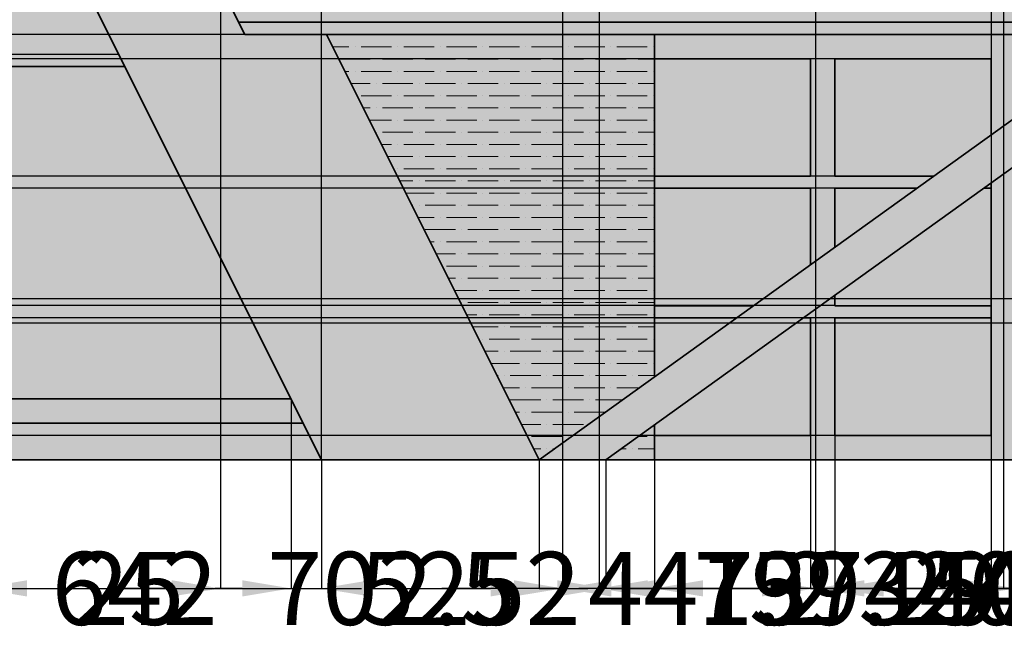
# Model space of a CAD drawing. Units: millimetres. Extents: x -504 to 6314, y 1290 to 4335.
# Tile 3 of 9: x 1774 to 3796, y 1290 to 2556. Entities that reach past the tile are written whole.
import ezdxf

# ---------------------------------------------------------------- set-up
doc = ezdxf.new("R2010")
doc.units = ezdxf.units.MM
doc.header["$MEASUREMENT"] = 0
for name, color, linetype, lineweight in [('A-ANNO-DIMS', 2, 'Continuous', 18), ('A-ELEV', 7, 'Continuous', 35), ('A-ELEV-PATT', 8, 'Continuous', 13)]:
    doc.layers.add(name, color=color, linetype=linetype, lineweight=lineweight)
doc.styles.get("Standard").update_dxf_attribs({"font": 'arial.ttf'})
doc.dimstyles.get("Standard").update_dxf_attribs({"dimtxt": 150, "dimasz": 100, "dimexe": 0.18, "dimexo": 0.0625, "dimgap": 0.09, "dimtad": 0, "dimtih": 1, "dimtoh": 1, "dimdec": 0, "dimzin": 0, "dimdsep": 46, "dimtxsty": 'Standard', "dimcen": 0.09, "dimadec": 0, "dimazin": 0, "dimtfac": 1, "dimtdec": 0, "dimtofl": 0, "dimtmove": 0, "dimatfit": 3, "dimfxl": 1, "dimtolj": 1, "dimtzin": 0, "dimarcsym": 0})
pattern_1 = [(50, (0, 0), (71.726, -6.2752), [7.5, -82.5]), (355, (0, 0), (-13.8751, 75.2192), [6, -66]), (100.4514, (5.98, -0.52), (57.8509, 68.944), [6.374, -70.1142]), (46.1842, (0, 20), (106.7241, -16.5519), [11.25, -123.75]), (96.6356, (8.89, 18.62), (93.4662, 97.4119), [9.561, -105.1714]), (351.1842, (0, 20), (93.4662, 97.4119), [9, -99]), (21, (10, 15), (59.6907, -40.2619), [7.5, -82.5]), (326, (10, 15), (24.3315, 72.515), [6, -66]), (71.4514, (14.974, 11.645), (84.0222, 32.2531), [6.374, -70.1142]), (37.5, (0, 0), (1.21599, 33.28939), [0, -65.2, 0, -67, 0, -66.25]), (7.5, (0, 0), (26.30695, 39.44117), [0, -38.2, 0, -63.7, 0, -25.25]), (327.5, (-22.3, 0), (53.38224, -2.25549), [0, -25, 0, -78, 0, -103.5]), (317.5, (-32.3, 0), (58.3186, 10.0105), [0, -32.5, 0, -51.8, 0, -73.5])]

# ---------------------------------------------------------------- blocks, each defined once
blk = doc.blocks.new('*D1')
at = {"layer": 'A-ANNO-DIMS', "color": 0, "lineweight": -2, "transparency": 16777216}
for p, q in [((5324.8, 2261.1), (5324.8, 1387.9)), ((72.8, 1652.1), (72.8, 1387.9)), ((172.8, 1388.1), (2475.5, 1388.1)), ((5224.8, 1388.1), (2922.1, 1388.1))]:
    blk.add_line(p, q, dxfattribs=at)
at = {"layer": 'A-ANNO-DIMS', "color": 0, "transparency": 16777216}
for points in [[(172.8, 1404.8), (172.8, 1371.5), (72.8, 1388.1)], [(5224.8, 1404.8), (5224.8, 1371.5), (5324.8, 1388.1)]]:
    blk.add_solid(points, dxfattribs=at)
at = {"layer": 'Defpoints', "color": 0, "transparency": 16777216}
for p in [(5324.8, 2261.2), (72.8, 1652.1), (5324.8, 1388.1)]:
    blk.add_point(p, dxfattribs=at)
at = {"layer": 'A-ANNO-DIMS', "color": 0, "transparency": 16777216, "insert": (2698.8, 1388.1), "char_height": 150, "attachment_point": 5}
blk.add_mtext('\\A1;5252', dxfattribs=at)
blk = doc.blocks.new('*D5')
at = {"layer": 'A-ANNO-DIMS', "color": 0, "lineweight": -2, "transparency": 16777216}
for p, q in [((4260.1, 2625.8), (5589, 2625.8)), ((5588.8, 2525.8), (5588.8, 2215.7)), ((5588.8, 1752.1), (5588.8, 2062.2)), ((72.9, 1652.1), (5589, 1652.1))]:
    blk.add_line(p, q, dxfattribs=at)
at = {"layer": 'A-ANNO-DIMS', "color": 0, "transparency": 16777216}
for points in [[(5572.1, 2525.8), (5605.5, 2525.8), (5588.8, 2625.8)], [(5572.1, 1752.1), (5605.5, 1752.1), (5588.8, 1652.1)]]:
    blk.add_solid(points, dxfattribs=at)
at = {"layer": 'Defpoints', "color": 0, "transparency": 16777216}
for p in [(4260, 2625.8), (5588.8, 2625.8), (72.8, 1652.1)]:
    blk.add_point(p, dxfattribs=at)
at = {"layer": 'A-ANNO-DIMS', "color": 0, "transparency": 16777216, "insert": (5588.8, 2138.9), "char_height": 150, "attachment_point": 5}
blk.add_mtext('\\A1;973.6', dxfattribs=at)
blk = doc.blocks.new('*D6')
at = {"layer": 'A-ANNO-DIMS', "color": 0, "lineweight": -2, "transparency": 16777216}
for p, q in [((72.8, 1652.2), (72.8, 4237)), ((172.8, 4236.8), (920.4, 4236.8)), ((2293.5, 4236.8), (1545.9, 4236.8)), ((2393.5, 1652.2), (2393.5, 4237))]:
    blk.add_line(p, q, dxfattribs=at)
at = {"layer": 'A-ANNO-DIMS', "color": 0, "transparency": 16777216}
for points in [[(172.8, 4253.4), (172.8, 4220.1), (72.8, 4236.8)], [(2293.5, 4253.4), (2293.5, 4220.1), (2393.5, 4236.8)]]:
    blk.add_solid(points, dxfattribs=at)
at = {"layer": 'Defpoints', "color": 0, "transparency": 16777216}
for p in [(2393.5, 4236.8), (72.8, 1652.1), (2393.5, 1652.1)]:
    blk.add_point(p, dxfattribs=at)
at = {"layer": 'A-ANNO-DIMS', "color": 0, "transparency": 16777216, "insert": (1233.2, 4236.8), "char_height": 150, "attachment_point": 5}
blk.add_mtext('\\A1;2320.7', dxfattribs=at)
blk = doc.blocks.new('*D12')
at = {"layer": 'A-ANNO-DIMS', "color": 0, "lineweight": -2, "transparency": 16777216}
for p, q in [((1664, 1777.1), (1664, 1387.9)), ((1689, 1777.1), (1689, 1387.9)), ((1564, 1388.1), (1464, 1388.1)), ((1789, 1388.1), (1889, 1388.1))]:
    blk.add_line(p, q, dxfattribs=at)
at = {"layer": 'A-ANNO-DIMS', "color": 0, "transparency": 16777216}
for points in [[(1564, 1404.8), (1564, 1371.5), (1664, 1388.1)], [(1789, 1404.8), (1789, 1371.5), (1689, 1388.1)]]:
    blk.add_solid(points, dxfattribs=at)
at = {"layer": 'Defpoints', "color": 0, "transparency": 16777216}
for p in [(1664, 1777.1), (1689, 1777.1), (1689, 1388.1)]:
    blk.add_point(p, dxfattribs=at)
at = {"layer": 'A-ANNO-DIMS', "color": 0, "transparency": 16777216, "insert": (1998.4, 1388.1), "char_height": 150, "attachment_point": 5}
blk.add_mtext('\\A1;25', dxfattribs=at)
blk = doc.blocks.new('*D13')
at = {"layer": 'A-ANNO-DIMS', "color": 0, "lineweight": -2, "transparency": 16777216}
for p, q in [((1689, 1777.1), (1689, 1387.9)), ((2331, 1777.1), (2331, 1387.9)), ((1789, 1388.1), (1844.6, 1388.1)), ((2231, 1388.1), (2175.4, 1388.1))]:
    blk.add_line(p, q, dxfattribs=at)
at = {"layer": 'A-ANNO-DIMS', "color": 0, "transparency": 16777216}
for points in [[(1789, 1404.8), (1789, 1371.5), (1689, 1388.1)], [(2231, 1404.8), (2231, 1371.5), (2331, 1388.1)]]:
    blk.add_solid(points, dxfattribs=at)
at = {"layer": 'Defpoints', "color": 0, "transparency": 16777216}
for p in [(1689, 1777.1), (2331, 1777.1), (2331, 1388.1)]:
    blk.add_point(p, dxfattribs=at)
at = {"layer": 'A-ANNO-DIMS', "color": 0, "transparency": 16777216, "insert": (2010, 1388.1), "char_height": 150, "attachment_point": 5}
blk.add_mtext('\\A1;642', dxfattribs=at)
blk = doc.blocks.new('*D36')
at = {"layer": 'A-ANNO-DIMS', "color": 0, "lineweight": -2, "transparency": 16777216}
for p, q in [((2186.2, 2625.7), (2186.2, 1387.9)), ((2888.6, 2625.7), (2888.6, 1387.9)), ((2086.2, 1388.1), (1986.2, 1388.1)), ((2988.6, 1388.1), (3088.6, 1388.1))]:
    blk.add_line(p, q, dxfattribs=at)
at = {"layer": 'A-ANNO-DIMS', "color": 0, "transparency": 16777216}
for points in [[(2086.2, 1404.8), (2086.2, 1371.5), (2186.2, 1388.1)], [(2988.6, 1404.8), (2988.6, 1371.5), (2888.6, 1388.1)]]:
    blk.add_solid(points, dxfattribs=at)
at = {"layer": 'Defpoints', "color": 0, "transparency": 16777216}
for p in [(2186.2, 2625.8), (2888.6, 2625.8), (2888.6, 1388.1)]:
    blk.add_point(p, dxfattribs=at)
at = {"layer": 'A-ANNO-DIMS', "color": 0, "transparency": 16777216, "insert": (2537.4, 1388.1), "char_height": 150, "attachment_point": 5}
blk.add_mtext('\\A1;702.5', dxfattribs=at)
blk = doc.blocks.new('*D37')
at = {"layer": 'A-ANNO-DIMS', "color": 0, "lineweight": -2, "transparency": 16777216}
for p, q in [((2888.6, 2625.7), (2888.6, 1387.9)), ((2963.6, 2625.7), (2963.6, 1387.9)), ((2788.6, 1388.1), (2688.6, 1388.1)), ((3063.6, 1388.1), (3163.6, 1388.1))]:
    blk.add_line(p, q, dxfattribs=at)
at = {"layer": 'A-ANNO-DIMS', "color": 0, "transparency": 16777216}
for points in [[(2788.6, 1404.8), (2788.6, 1371.5), (2888.6, 1388.1)], [(3063.6, 1404.8), (3063.6, 1371.5), (2963.6, 1388.1)]]:
    blk.add_solid(points, dxfattribs=at)
at = {"layer": 'Defpoints', "color": 0, "transparency": 16777216}
for p in [(2888.6, 2625.8), (2963.6, 2625.8), (2963.6, 1388.1)]:
    blk.add_point(p, dxfattribs=at)
at = {"layer": 'A-ANNO-DIMS', "color": 0, "transparency": 16777216, "insert": (3271.1, 1388.1), "char_height": 150, "attachment_point": 5}
blk.add_mtext('\\A1;75', dxfattribs=at)
blk = doc.blocks.new('*D38')
at = {"layer": 'A-ANNO-DIMS', "color": 0, "lineweight": -2, "transparency": 16777216}
for p, q in [((2963.6, 2625.7), (2963.6, 1387.9)), ((3407.8, 2625.7), (3407.8, 1387.9)), ((3063.6, 1388.1), (3307.8, 1388.1)), ((3407.8, 1388.1), (3507.8, 1388.1))]:
    blk.add_line(p, q, dxfattribs=at)
at = {"layer": 'A-ANNO-DIMS', "color": 0, "transparency": 16777216}
for points in [[(3063.6, 1404.8), (3063.6, 1371.5), (2963.6, 1388.1)], [(3307.8, 1404.8), (3307.8, 1371.5), (3407.8, 1388.1)]]:
    blk.add_solid(points, dxfattribs=at)
at = {"layer": 'Defpoints', "color": 0, "transparency": 16777216}
for p in [(2963.6, 2625.8), (3407.8, 2625.8), (3407.8, 1388.1)]:
    blk.add_point(p, dxfattribs=at)
at = {"layer": 'A-ANNO-DIMS', "color": 0, "transparency": 16777216, "insert": (3763.2, 1388.1), "char_height": 150, "attachment_point": 5}
blk.add_mtext('\\A1;444.2', dxfattribs=at)
blk = doc.blocks.new('*D39')
at = {"layer": 'A-ANNO-DIMS', "color": 0, "lineweight": -2, "transparency": 16777216}
for p, q in [((3407.8, 2625.7), (3407.8, 1387.9)), ((3768.6, 2625.7), (3768.6, 1387.9)), ((3507.8, 1388.1), (3668.6, 1388.1)), ((3768.6, 1388.1), (3868.6, 1388.1))]:
    blk.add_line(p, q, dxfattribs=at)
at = {"layer": 'A-ANNO-DIMS', "color": 0, "transparency": 16777216}
for points in [[(3507.8, 1404.8), (3507.8, 1371.5), (3407.8, 1388.1)], [(3668.6, 1404.8), (3668.6, 1371.5), (3768.6, 1388.1)]]:
    blk.add_solid(points, dxfattribs=at)
at = {"layer": 'Defpoints', "color": 0, "transparency": 16777216}
for p in [(3407.8, 2625.8), (3768.6, 2625.8), (3768.6, 1388.1)]:
    blk.add_point(p, dxfattribs=at)
at = {"layer": 'A-ANNO-DIMS', "color": 0, "transparency": 16777216, "insert": (4179.7, 1388.1), "char_height": 150, "attachment_point": 5}
blk.add_mtext('\\A1;360.84', dxfattribs=at)
blk = doc.blocks.new('*D40')
at = {"layer": 'A-ANNO-DIMS', "color": 0, "lineweight": -2, "transparency": 16777216}
for p, q in [((3768.6, 2625.7), (3768.6, 1387.9)), ((3793.6, 2625.7), (3793.6, 1387.9)), ((3668.6, 1388.1), (3568.6, 1388.1)), ((3893.6, 1388.1), (3993.6, 1388.1))]:
    blk.add_line(p, q, dxfattribs=at)
at = {"layer": 'A-ANNO-DIMS', "color": 0, "transparency": 16777216}
for points in [[(3668.6, 1404.8), (3668.6, 1371.5), (3768.6, 1388.1)], [(3893.6, 1404.8), (3893.6, 1371.5), (3793.6, 1388.1)]]:
    blk.add_solid(points, dxfattribs=at)
at = {"layer": 'Defpoints', "color": 0, "transparency": 16777216}
for p in [(3768.6, 2625.8), (3793.6, 2625.8), (3793.6, 1388.1)]:
    blk.add_point(p, dxfattribs=at)
at = {"layer": 'A-ANNO-DIMS', "color": 0, "transparency": 16777216, "insert": (4103, 1388.1), "char_height": 150, "attachment_point": 5}
blk.add_mtext('\\A1;25', dxfattribs=at)
blk = doc.blocks.new('*D41')
at = {"layer": 'A-ANNO-DIMS', "color": 0, "lineweight": -2, "transparency": 16777216}
for p, q in [((3793.6, 2625.7), (3793.6, 1387.9)), ((3818.6, 2625.7), (3818.6, 1387.9)), ((3693.6, 1388.1), (3593.6, 1388.1)), ((3918.6, 1388.1), (4018.6, 1388.1))]:
    blk.add_line(p, q, dxfattribs=at)
at = {"layer": 'A-ANNO-DIMS', "color": 0, "transparency": 16777216}
for points in [[(3693.6, 1404.8), (3693.6, 1371.5), (3793.6, 1388.1)], [(3918.6, 1404.8), (3918.6, 1371.5), (3818.6, 1388.1)]]:
    blk.add_solid(points, dxfattribs=at)
at = {"layer": 'Defpoints', "color": 0, "transparency": 16777216}
for p in [(3793.6, 2625.8), (3818.6, 2625.8), (3818.6, 1388.1)]:
    blk.add_point(p, dxfattribs=at)
at = {"layer": 'A-ANNO-DIMS', "color": 0, "transparency": 16777216, "insert": (4128, 1388.1), "char_height": 150, "attachment_point": 5}
blk.add_mtext('\\A1;25', dxfattribs=at)
blk = doc.blocks.new('*D42')
at = {"layer": 'A-ANNO-DIMS', "color": 0, "lineweight": -2, "transparency": 16777216}
for p, q in [((3818.6, 2625.7), (3818.6, 1387.9)), ((4198.6, 2625.7), (4198.6, 1387.9)), ((3718.6, 1388.1), (3618.6, 1388.1)), ((4298.6, 1388.1), (4398.6, 1388.1))]:
    blk.add_line(p, q, dxfattribs=at)
at = {"layer": 'A-ANNO-DIMS', "color": 0, "transparency": 16777216}
for points in [[(3718.6, 1404.8), (3718.6, 1371.5), (3818.6, 1388.1)], [(4298.6, 1404.8), (4298.6, 1371.5), (4198.6, 1388.1)]]:
    blk.add_solid(points, dxfattribs=at)
at = {"layer": 'Defpoints', "color": 0, "transparency": 16777216}
for p in [(3818.6, 2625.8), (4198.6, 2625.8), (4198.6, 1388.1)]:
    blk.add_point(p, dxfattribs=at)
at = {"layer": 'A-ANNO-DIMS', "color": 0, "transparency": 16777216, "insert": (4008.6, 1388.1), "char_height": 150, "attachment_point": 5}
blk.add_mtext('\\A1;380', dxfattribs=at)
blk = doc.blocks.new('*D48')
at = {"layer": 'A-ANNO-DIMS', "color": 0, "lineweight": -2, "transparency": 16777216}
for p, q in [((2393.5, 1652.1), (2393.5, 1387.9)), ((2840.7, 1652.1), (2840.7, 1387.9)), ((2493.5, 1388.1), (2740.7, 1388.1)), ((2840.7, 1388.1), (2940.7, 1388.1))]:
    blk.add_line(p, q, dxfattribs=at)
at = {"layer": 'A-ANNO-DIMS', "color": 0, "transparency": 16777216}
for points in [[(2493.5, 1404.8), (2493.5, 1371.5), (2393.5, 1388.1)], [(2740.7, 1404.8), (2740.7, 1371.5), (2840.7, 1388.1)]]:
    blk.add_solid(points, dxfattribs=at)
at = {"layer": 'Defpoints', "color": 0, "transparency": 16777216}
for p in [(2393.5, 1652.1), (2840.7, 1652.1), (2840.7, 1388.1)]:
    blk.add_point(p, dxfattribs=at)
at = {"layer": 'A-ANNO-DIMS', "color": 0, "transparency": 16777216, "insert": (3196.1, 1388.1), "char_height": 150, "attachment_point": 5}
blk.add_mtext('\\A1;447.2', dxfattribs=at)
blk = doc.blocks.new('*D49')
at = {"layer": 'A-ANNO-DIMS', "color": 0, "lineweight": -2, "transparency": 16777216}
for p, q in [((2840.7, 1652.1), (2840.7, 1387.9)), ((2977.7, 1652.1), (2977.7, 1387.9)), ((2740.7, 1388.1), (2640.7, 1388.1)), ((3077.7, 1388.1), (3177.7, 1388.1))]:
    blk.add_line(p, q, dxfattribs=at)
at = {"layer": 'A-ANNO-DIMS', "color": 0, "transparency": 16777216}
for points in [[(2740.7, 1404.8), (2740.7, 1371.5), (2840.7, 1388.1)], [(3077.7, 1404.8), (3077.7, 1371.5), (2977.7, 1388.1)]]:
    blk.add_solid(points, dxfattribs=at)
at = {"layer": 'Defpoints', "color": 0, "transparency": 16777216}
for p in [(2840.7, 1652.1), (2977.7, 1652.1), (2977.7, 1388.1)]:
    blk.add_point(p, dxfattribs=at)
at = {"layer": 'A-ANNO-DIMS', "color": 0, "transparency": 16777216, "insert": (3336.4, 1388.1), "char_height": 150, "attachment_point": 5}
blk.add_mtext('\\A1;137', dxfattribs=at)
blk = doc.blocks.new('*D50')
at = {"layer": 'A-ANNO-DIMS', "color": 0, "lineweight": -2, "transparency": 16777216}
for p, q in [((3077, 1702.1), (3077, 1387.9)), ((2977.7, 1652.1), (2977.7, 1387.9)), ((2877.7, 1388.1), (2777.7, 1388.1)), ((3177, 1388.1), (3277, 1388.1))]:
    blk.add_line(p, q, dxfattribs=at)
at = {"layer": 'A-ANNO-DIMS', "color": 0, "transparency": 16777216}
for points in [[(2877.7, 1404.8), (2877.7, 1371.5), (2977.7, 1388.1)], [(3177, 1404.8), (3177, 1371.5), (3077, 1388.1)]]:
    blk.add_solid(points, dxfattribs=at)
at = {"layer": 'Defpoints', "color": 0, "transparency": 16777216}
for p in [(3077, 1702.1), (2977.7, 1652.1), (3077, 1388.1)]:
    blk.add_point(p, dxfattribs=at)
at = {"layer": 'A-ANNO-DIMS', "color": 0, "transparency": 16777216, "insert": (3530.3, 1388.1), "char_height": 150, "attachment_point": 5}
blk.add_mtext('\\A1;99.29', dxfattribs=at)
blk = doc.blocks.new('*D51')
at = {"layer": 'A-ANNO-DIMS', "color": 0, "lineweight": -2, "transparency": 16777216}
for p, q in [((3077, 1702.1), (3077, 1387.9)), ((3397.8, 1702.1), (3397.8, 1387.9)), ((3177, 1388.1), (3297.8, 1388.1)), ((3397.8, 1388.1), (3497.8, 1388.1))]:
    blk.add_line(p, q, dxfattribs=at)
at = {"layer": 'A-ANNO-DIMS', "color": 0, "transparency": 16777216}
for points in [[(3177, 1404.8), (3177, 1371.5), (3077, 1388.1)], [(3297.8, 1404.8), (3297.8, 1371.5), (3397.8, 1388.1)]]:
    blk.add_solid(points, dxfattribs=at)
at = {"layer": 'Defpoints', "color": 0, "transparency": 16777216}
for p in [(3077, 1702.1), (3397.8, 1702.1), (3397.8, 1388.1)]:
    blk.add_point(p, dxfattribs=at)
at = {"layer": 'A-ANNO-DIMS', "color": 0, "transparency": 16777216, "insert": (3751.1, 1388.1), "char_height": 150, "attachment_point": 5}
blk.add_mtext('\\A1;320.8', dxfattribs=at)
blk = doc.blocks.new('*D52')
at = {"layer": 'A-ANNO-DIMS', "color": 0, "lineweight": -2, "transparency": 16777216}
for p, q in [((3397.8, 1702.1), (3397.8, 1387.9)), ((3447.8, 1702.1), (3447.8, 1387.9)), ((3297.8, 1388.1), (3197.8, 1388.1)), ((3547.8, 1388.1), (3647.8, 1388.1))]:
    blk.add_line(p, q, dxfattribs=at)
at = {"layer": 'A-ANNO-DIMS', "color": 0, "transparency": 16777216}
for points in [[(3297.8, 1404.8), (3297.8, 1371.5), (3397.8, 1388.1)], [(3547.8, 1404.8), (3547.8, 1371.5), (3447.8, 1388.1)]]:
    blk.add_solid(points, dxfattribs=at)
at = {"layer": 'Defpoints', "color": 0, "transparency": 16777216}
for p in [(3397.8, 1702.1), (3447.8, 1702.1), (3447.8, 1388.1)]:
    blk.add_point(p, dxfattribs=at)
at = {"layer": 'A-ANNO-DIMS', "color": 0, "transparency": 16777216, "insert": (3755.1, 1388.1), "char_height": 150, "attachment_point": 5}
blk.add_mtext('\\A1;50', dxfattribs=at)
blk = doc.blocks.new('*D53')
at = {"layer": 'A-ANNO-DIMS', "color": 0, "lineweight": -2, "transparency": 16777216}
for p, q in [((3447.8, 1702.1), (3447.8, 1387.9)), ((3768.6, 1702.1), (3768.6, 1387.9)), ((3547.8, 1388.1), (3668.6, 1388.1)), ((3768.6, 1388.1), (3868.6, 1388.1))]:
    blk.add_line(p, q, dxfattribs=at)
at = {"layer": 'A-ANNO-DIMS', "color": 0, "transparency": 16777216}
for points in [[(3547.8, 1404.8), (3547.8, 1371.5), (3447.8, 1388.1)], [(3668.6, 1404.8), (3668.6, 1371.5), (3768.6, 1388.1)]]:
    blk.add_solid(points, dxfattribs=at)
at = {"layer": 'Defpoints', "color": 0, "transparency": 16777216}
for p in [(3447.8, 1702.1), (3768.6, 1702.1), (3768.6, 1388.1)]:
    blk.add_point(p, dxfattribs=at)
at = {"layer": 'A-ANNO-DIMS', "color": 0, "transparency": 16777216, "insert": (4121.9, 1388.1), "char_height": 150, "attachment_point": 5}
blk.add_mtext('\\A1;320.8', dxfattribs=at)
blk = doc.blocks.new('*D54')
at = {"layer": 'A-ANNO-DIMS', "color": 0, "lineweight": -2, "transparency": 16777216}
for p, q in [((3768.6, 1702.1), (3768.6, 1387.9)), ((3818.6, 1652.1), (3818.6, 1387.9)), ((3668.6, 1388.1), (3568.6, 1388.1)), ((3918.6, 1388.1), (4018.6, 1388.1))]:
    blk.add_line(p, q, dxfattribs=at)
at = {"layer": 'A-ANNO-DIMS', "color": 0, "transparency": 16777216}
for points in [[(3668.6, 1404.8), (3668.6, 1371.5), (3768.6, 1388.1)], [(3918.6, 1404.8), (3918.6, 1371.5), (3818.6, 1388.1)]]:
    blk.add_solid(points, dxfattribs=at)
at = {"layer": 'Defpoints', "color": 0, "transparency": 16777216}
for p in [(3768.6, 1702.1), (3818.6, 1652.1), (3818.6, 1388.1)]:
    blk.add_point(p, dxfattribs=at)
at = {"layer": 'A-ANNO-DIMS', "color": 0, "transparency": 16777216, "insert": (4125.9, 1388.1), "char_height": 150, "attachment_point": 5}
blk.add_mtext('\\A1;50', dxfattribs=at)
blk = doc.blocks.new('*D55')
at = {"layer": 'A-ANNO-DIMS', "color": 0, "lineweight": -2, "transparency": 16777216}
for p, q in [((3818.6, 1652.1), (3818.6, 1387.9)), ((3997.4, 1652.1), (3997.4, 1387.9)), ((3718.6, 1388.1), (3618.6, 1388.1)), ((4097.4, 1388.1), (4197.4, 1388.1))]:
    blk.add_line(p, q, dxfattribs=at)
at = {"layer": 'A-ANNO-DIMS', "color": 0, "transparency": 16777216}
for points in [[(3718.6, 1404.8), (3718.6, 1371.5), (3818.6, 1388.1)], [(4097.4, 1404.8), (4097.4, 1371.5), (3997.4, 1388.1)]]:
    blk.add_solid(points, dxfattribs=at)
at = {"layer": 'Defpoints', "color": 0, "transparency": 16777216}
for p in [(3818.6, 1652.1), (3997.4, 1652.1), (3997.4, 1388.1)]:
    blk.add_point(p, dxfattribs=at)
at = {"layer": 'A-ANNO-DIMS', "color": 0, "transparency": 16777216, "insert": (4502.3, 1388.1), "char_height": 150, "attachment_point": 5}
blk.add_mtext('\\A1;178.75', dxfattribs=at)
blk = doc.blocks.new('*D66')
at = {"layer": 'A-ANNO-DIMS', "color": 0, "lineweight": -2, "transparency": 16777216}
for p, q in [((3753.7, 4236.8), (3653.7, 4236.8)), ((3853.7, 1932.9), (3853.7, 4237)), ((3992.1, 1982.9), (3992.1, 4237)), ((4092.1, 4236.8), (4192.1, 4236.8))]:
    blk.add_line(p, q, dxfattribs=at)
at = {"layer": 'A-ANNO-DIMS', "color": 0, "transparency": 16777216}
for points in [[(3753.7, 4253.4), (3753.7, 4220.1), (3853.7, 4236.8)], [(4092.1, 4253.4), (4092.1, 4220.1), (3992.1, 4236.8)]]:
    blk.add_solid(points, dxfattribs=at)
at = {"layer": 'Defpoints', "color": 0, "transparency": 16777216}
for p in [(3992.1, 4236.8), (3992.1, 1982.8), (3853.7, 1932.8)]:
    blk.add_point(p, dxfattribs=at)
at = {"layer": 'A-ANNO-DIMS', "color": 0, "transparency": 16777216, "insert": (4496.6, 4236.8), "char_height": 150, "attachment_point": 5}
blk.add_mtext('\\A1;138.38', dxfattribs=at)
blk = doc.blocks.new('*D67')
at = {"layer": 'A-ANNO-DIMS', "color": 0, "lineweight": -2, "transparency": 16777216}
for p, q in [((-191.2, 2082.8), (-191.2, 2182.8)), ((-191.2, 2182.8), (-91.2, 2182.8)), ((3992, 1982.8), (-191.3, 1982.8)), ((3853.6, 1932.8), (-191.3, 1932.8)), ((-191.2, 1832.8), (-191.2, 1732.8))]:
    blk.add_line(p, q, dxfattribs=at)
at = {"layer": 'A-ANNO-DIMS', "color": 0, "transparency": 16777216}
for points in [[(-207.8, 2082.8), (-174.5, 2082.8), (-191.2, 1982.8)], [(-207.8, 1832.8), (-174.5, 1832.8), (-191.2, 1932.8)]]:
    blk.add_solid(points, dxfattribs=at)
at = {"layer": 'Defpoints', "color": 0, "transparency": 16777216}
for p in [(-191.2, 1982.8), (3992.1, 1982.8), (3853.7, 1932.8)]:
    blk.add_point(p, dxfattribs=at)
at = {"layer": 'A-ANNO-DIMS', "color": 0, "transparency": 16777216, "insert": (16.1, 2182.8), "char_height": 150, "attachment_point": 5}
blk.add_mtext('\\A1;50', dxfattribs=at)
blk = doc.blocks.new('*D68')
at = {"layer": 'A-ANNO-DIMS', "color": 0, "lineweight": -2, "transparency": 16777216}
for p, q in [((-191.2, 1802.1), (-191.2, 1902.1)), ((-191.2, 1902.1), (-91.2, 1902.1)), ((3076.9, 1702.1), (-191.3, 1702.1)), ((3076.9, 1652.1), (-191.3, 1652.1)), ((-191.2, 1552.1), (-191.2, 1452.1))]:
    blk.add_line(p, q, dxfattribs=at)
at = {"layer": 'A-ANNO-DIMS', "color": 0, "transparency": 16777216}
for points in [[(-207.8, 1802.1), (-174.5, 1802.1), (-191.2, 1702.1)], [(-207.8, 1552.1), (-174.5, 1552.1), (-191.2, 1652.1)]]:
    blk.add_solid(points, dxfattribs=at)
at = {"layer": 'Defpoints', "color": 0, "transparency": 16777216}
for p in [(-191.2, 1702.1), (3077, 1702.1), (3077, 1652.1)]:
    blk.add_point(p, dxfattribs=at)
at = {"layer": 'A-ANNO-DIMS', "color": 0, "transparency": 16777216, "insert": (16.1, 1902.1), "char_height": 150, "attachment_point": 5}
blk.add_mtext('\\A1;50', dxfattribs=at)
blk = doc.blocks.new('*D69')
at = {"layer": 'A-ANNO-DIMS', "color": 0, "lineweight": -2, "transparency": 16777216}
for p, q in [((-191.2, 2625.8), (-191.2, 2725.8)), ((-191.2, 2725.8), (-91.2, 2725.8)), ((3076.9, 2525.8), (-191.3, 2525.8)), ((3076.9, 2475.8), (-191.3, 2475.8)), ((-191.2, 2375.8), (-191.2, 2275.8))]:
    blk.add_line(p, q, dxfattribs=at)
at = {"layer": 'A-ANNO-DIMS', "color": 0, "transparency": 16777216}
for points in [[(-207.8, 2625.8), (-174.5, 2625.8), (-191.2, 2525.8)], [(-207.8, 2375.8), (-174.5, 2375.8), (-191.2, 2475.8)]]:
    blk.add_solid(points, dxfattribs=at)
at = {"layer": 'Defpoints', "color": 0, "transparency": 16777216}
for p in [(-191.2, 2525.8), (3077, 2525.8), (3077, 2475.8)]:
    blk.add_point(p, dxfattribs=at)
at = {"layer": 'A-ANNO-DIMS', "color": 0, "transparency": 16777216, "insert": (16.1, 2725.8), "char_height": 150, "attachment_point": 5}
blk.add_mtext('\\A1;50', dxfattribs=at)
blk = doc.blocks.new('*D70')
at = {"layer": 'A-ANNO-DIMS', "color": 0, "lineweight": -2, "transparency": 16777216}
for p, q in [((-191.2, 1943.8), (-191.2, 2043.8)), ((-191.2, 2043.8), (-91.2, 2043.8)), ((3447.7, 1943.8), (-191.3, 1943.8)), ((-191.2, 1802.1), (-191.2, 1843.8)), ((3447.7, 1702.1), (-191.3, 1702.1))]:
    blk.add_line(p, q, dxfattribs=at)
at = {"layer": 'A-ANNO-DIMS', "color": 0, "transparency": 16777216}
for points in [[(-207.8, 1843.8), (-174.5, 1843.8), (-191.2, 1943.8)], [(-207.8, 1802.1), (-174.5, 1802.1), (-191.2, 1702.1)]]:
    blk.add_solid(points, dxfattribs=at)
at = {"layer": 'Defpoints', "color": 0, "transparency": 16777216}
for p in [(-191.2, 1943.8), (3447.8, 1943.8), (3447.8, 1702.1)]:
    blk.add_point(p, dxfattribs=at)
at = {"layer": 'A-ANNO-DIMS', "color": 0, "transparency": 16777216, "insert": (221.6, 2043.8), "char_height": 150, "attachment_point": 5}
blk.add_mtext('\\A1;241.63', dxfattribs=at)
blk = doc.blocks.new('*D71')
at = {"layer": 'A-ANNO-DIMS', "color": 0, "lineweight": -2, "transparency": 16777216}
for p, q in [((-191.2, 2068.8), (-191.2, 2168.8)), ((-191.2, 2168.8), (-91.2, 2168.8)), ((3447.7, 1968.8), (-191.3, 1968.8)), ((3447.7, 1943.8), (-191.3, 1943.8)), ((-191.2, 1843.8), (-191.2, 1743.8))]:
    blk.add_line(p, q, dxfattribs=at)
at = {"layer": 'A-ANNO-DIMS', "color": 0, "transparency": 16777216}
for points in [[(-207.8, 2068.8), (-174.5, 2068.8), (-191.2, 1968.8)], [(-207.8, 1843.8), (-174.5, 1843.8), (-191.2, 1943.8)]]:
    blk.add_solid(points, dxfattribs=at)
at = {"layer": 'Defpoints', "color": 0, "transparency": 16777216}
for p in [(-191.2, 1968.8), (3447.8, 1968.8), (3447.8, 1943.8)]:
    blk.add_point(p, dxfattribs=at)
at = {"layer": 'A-ANNO-DIMS', "color": 0, "transparency": 16777216, "insert": (18.2, 2168.8), "char_height": 150, "attachment_point": 5}
blk.add_mtext('\\A1;25', dxfattribs=at)
blk = doc.blocks.new('*D72')
at = {"layer": 'A-ANNO-DIMS', "color": 0, "lineweight": -2, "transparency": 16777216}
for p, q in [((-191.2, 2209.8), (-191.2, 2309.8)), ((-191.2, 2309.8), (-91.2, 2309.8)), ((3447.7, 2209.8), (-191.3, 2209.8)), ((-191.2, 2068.8), (-191.2, 2109.8)), ((3447.7, 1968.8), (-191.3, 1968.8))]:
    blk.add_line(p, q, dxfattribs=at)
at = {"layer": 'A-ANNO-DIMS', "color": 0, "transparency": 16777216}
for points in [[(-207.8, 2109.8), (-174.5, 2109.8), (-191.2, 2209.8)], [(-207.8, 2068.8), (-174.5, 2068.8), (-191.2, 1968.8)]]:
    blk.add_solid(points, dxfattribs=at)
at = {"layer": 'Defpoints', "color": 0, "transparency": 16777216}
for p in [(-191.2, 2209.8), (3447.8, 2209.8), (3447.8, 1968.8)]:
    blk.add_point(p, dxfattribs=at)
at = {"layer": 'A-ANNO-DIMS', "color": 0, "transparency": 16777216, "insert": (61.4, 2309.8), "char_height": 150, "attachment_point": 5}
blk.add_mtext('\\A1;241', dxfattribs=at)
blk = doc.blocks.new('*D73')
at = {"layer": 'A-ANNO-DIMS', "color": 0, "lineweight": -2, "transparency": 16777216}
for p, q in [((-191.2, 2334.8), (-191.2, 2434.8)), ((-191.2, 2434.8), (-91.2, 2434.8)), ((3447.7, 2234.8), (-191.3, 2234.8)), ((3447.7, 2209.8), (-191.3, 2209.8)), ((-191.2, 2109.8), (-191.2, 2009.8))]:
    blk.add_line(p, q, dxfattribs=at)
at = {"layer": 'A-ANNO-DIMS', "color": 0, "transparency": 16777216}
for points in [[(-207.8, 2334.8), (-174.5, 2334.8), (-191.2, 2234.8)], [(-207.8, 2109.8), (-174.5, 2109.8), (-191.2, 2209.8)]]:
    blk.add_solid(points, dxfattribs=at)
at = {"layer": 'Defpoints', "color": 0, "transparency": 16777216}
for p in [(-191.2, 2234.8), (3447.8, 2234.8), (3447.8, 2209.8)]:
    blk.add_point(p, dxfattribs=at)
at = {"layer": 'A-ANNO-DIMS', "color": 0, "transparency": 16777216, "insert": (18.2, 2434.8), "char_height": 150, "attachment_point": 5}
blk.add_mtext('\\A1;25', dxfattribs=at)
blk = doc.blocks.new('*D74')
at = {"layer": 'A-ANNO-DIMS', "color": 0, "lineweight": -2, "transparency": 16777216}
for p, q in [((-191.2, 2475.8), (-191.2, 2575.8)), ((-191.2, 2575.8), (-91.2, 2575.8)), ((3447.7, 2475.8), (-191.3, 2475.8)), ((-191.2, 2334.8), (-191.2, 2375.8)), ((3447.7, 2234.8), (-191.3, 2234.8))]:
    blk.add_line(p, q, dxfattribs=at)
at = {"layer": 'A-ANNO-DIMS', "color": 0, "transparency": 16777216}
for points in [[(-207.8, 2375.8), (-174.5, 2375.8), (-191.2, 2475.8)], [(-207.8, 2334.8), (-174.5, 2334.8), (-191.2, 2234.8)]]:
    blk.add_solid(points, dxfattribs=at)
at = {"layer": 'Defpoints', "color": 0, "transparency": 16777216}
for p in [(-191.2, 2475.8), (3447.8, 2475.8), (3447.8, 2234.8)]:
    blk.add_point(p, dxfattribs=at)
at = {"layer": 'A-ANNO-DIMS', "color": 0, "transparency": 16777216, "insert": (61.4, 2575.8), "char_height": 150, "attachment_point": 5}
blk.add_mtext('\\A1;241', dxfattribs=at)

msp = doc.modelspace()

# ---------------------------------------------------------------- hatches: boundary and pattern name
at = {"layer": 'A-ELEV-PATT'}
for points in [[(3324.48, 3780.626), (1233.163, 3972.781), (72.835, 1652.125), (2393.491, 1652.125), (2355.991, 1727.125), (138.286, 1727.125), (1247.138, 3944.83), (2393.491, 1652.125), (2840.705, 1652.125), (2403.888, 2525.758), (2236.182, 2525.758), (2186.182, 2625.758), (2309.166, 2625.758), (1976.702, 3290.687), (1853.718, 3290.687), (1778.718, 3440.687), (3407.797, 3440.687)], [(1330.991, 3777.125), (1303.04, 3833.026), (250.089, 1727.125), (2355.991, 1727.125), (2330.991, 1777.125), (330.991, 1777.125)], [(1977.097, 2484.912), (1688.991, 2485.278), (1688.991, 3061.125), (1663.991, 3111.125), (1663.991, 2485.31), (1022.991, 2486.124), (1022.991, 3136.125), (1651.89, 3135.326), (1639.382, 3160.342), (1022.991, 3161.125), (997.991, 3111.125), (997.991, 2486.156), (685.705, 2486.552), (673.213, 2461.568), (997.991, 2461.156), (997.991, 1777.125), (1022.991, 1777.125), (1022.991, 2461.124), (1663.991, 2460.31), (1663.991, 1777.125), (1688.991, 1777.125), (1688.991, 2460.278), (1989.605, 2459.896)], [(5324.792, 2261.16), (5324.792, 2338.836), (4260.021, 2625.758), (3929.687, 2625.758), (3407.797, 2625.758), (2186.182, 2625.758), (2223.682, 2550.758), (3407.797, 2550.758), (3929.687, 2550.758), (4250.093, 2550.758)], [(4250.093, 2550.758), (3929.687, 2550.758), (3407.797, 2550.758), (2223.682, 2550.758), (2236.182, 2525.758), (3407.797, 2525.758), (3929.687, 2525.758), (4246.784, 2525.758), (5078.405, 2301.662), (3976.669, 2370.761), (3944.641, 2347.72), (5324.792, 2261.16)], [(3076.987, 1723.551), (2977.698, 1652.125), (3076.987, 1652.125)]]:
    msp.add_hatch(color=256, dxfattribs=at).paths.add_polyline_path(points)
h = msp.add_hatch(dxfattribs=at)
h.set_pattern_fill('ANSI36', color=256, scale=200, angle=135, style=0)
h.paths.add_polyline_path([(3324.48, 3780.626), (1233.163, 3972.781), (72.835, 1652.125), (2393.491, 1652.125), (2355.991, 1727.125), (138.286, 1727.125), (1247.138, 3944.83), (2393.491, 1652.125), (2840.705, 1652.125), (2403.888, 2525.758), (2236.182, 2525.758), (2186.182, 2625.758), (2309.166, 2625.758), (1976.702, 3290.687), (1853.718, 3290.687), (1778.718, 3440.687), (3407.797, 3440.687)])
h = msp.add_hatch(dxfattribs=at)
h.set_pattern_fill('AR-CONC', color=256, scale=10, style=0)
h.set_pattern_definition(pattern_1)
h.paths.add_polyline_path([(4308.57, 3440.687), (3929.687, 3440.687), (3407.797, 3440.687), (1778.718, 3440.687), (1828.718, 3340.687), (3407.797, 3340.687), (3929.687, 3340.687), (4304.463, 3340.687), (5081.168, 3138.941), (5082.876, 3139.564), (5082.876, 3239.564)])
h.paths.add_polyline_path([(4260.021, 2625.758), (3929.687, 2625.758), (3407.797, 2625.758), (2186.182, 2625.758), (2223.682, 2550.758), (3407.797, 2550.758), (3929.687, 2550.758), (4250.093, 2550.758), (5324.792, 2261.16), (5324.792, 2338.836)])
h = msp.add_hatch(color=256, dxfattribs=at)
h.set_gradient(color1=(99, 100, 102), color2=(254, 204, 102), name='CYLINDER')
h.paths.add_polyline_path([(1688.991, 3061.125), (1688.991, 2485.278), (1977.097, 2484.912)])
h.paths.add_polyline_path([(997.991, 3111.125), (685.705, 2486.552), (997.991, 2486.156)])
h = msp.add_hatch(color=256, dxfattribs=at)
h.set_gradient(color1=(147, 149, 152), color2=(254, 204, 102), tint=1, name='HEMISPHERICAL')
h.paths.add_polyline_path([(1688.991, 3061.125), (1688.991, 2485.278), (1977.097, 2484.912)])
h = msp.add_hatch(dxfattribs=at)
h.set_pattern_fill('AR-CONC', color=256, scale=10, style=0)
h.set_pattern_definition(pattern_1)
h.paths.add_polyline_path([(4260.021, 2625.758), (3929.687, 2625.758), (3407.797, 2625.758), (2186.182, 2625.758), (2223.682, 2550.758), (3407.797, 2550.758), (3929.687, 2550.758), (4250.093, 2550.758), (5324.792, 2261.16), (5324.792, 2338.836)])
h = msp.add_hatch(color=256, dxfattribs=at)
h.paths.add_polyline_path([(3076.987, 2525.758), (2403.888, 2525.758), (2840.705, 1652.125), (3076.987, 1822.101)])
h.paths.add_polyline_path([(3922.329, 1726.72), (3818.634, 1652.125), (3997.385, 1652.125)])
h.paths.add_polyline_path([(3818.634, 1829.779), (3818.634, 1738.093), (3872.15, 1776.591)])
h = msp.add_hatch(dxfattribs=at)
h.set_pattern_fill('ANSI36', color=256, scale=200, angle=135, style=0)
h.paths.add_polyline_path([(3076.987, 2525.758), (2403.888, 2525.758), (2840.705, 1652.125), (3076.987, 1822.101)])
h = msp.add_hatch(color=256, dxfattribs=at)
h.paths.add_polyline_path([(4192.131, 2525.758), (4055.138, 2525.758), (2840.705, 1652.125), (2977.698, 1652.125)])
h.paths.add_polyline_path([(4718.141, 2299.208), (4608.219, 2306.102), (3872.15, 1776.591), (3922.329, 1726.72)])
h = msp.add_hatch(color=256, dxfattribs=at)
h.paths.add_polyline_path([(3447.81, 1943.758), (3768.634, 1943.758), (3768.634, 1968.758), (3447.81, 1968.758), (3447.81, 1990.312), (3383.096, 1943.758), (3397.81, 1943.758), (3397.81, 1702.125), (3076.987, 1702.125), (3076.987, 1652.125), (3818.634, 1652.125), (3818.634, 2257.074), (3768.634, 2221.105), (3768.634, 1702.125), (3447.81, 1702.125)])
h.paths.add_polyline_path([(3650.62, 2234.758), (3447.81, 2234.758), (3447.81, 2475.758), (3768.634, 2475.758), (3768.634, 2319.654), (3818.634, 2355.623), (3818.634, 2525.758), (3407.797, 2525.758), (3076.987, 2525.758), (3076.987, 2475.758), (3397.81, 2475.758), (3397.81, 2234.758), (3076.987, 2234.758), (3076.987, 2209.758), (3397.81, 2209.758), (3397.81, 2052.893), (3447.81, 2088.862), (3447.81, 2209.758), (3615.868, 2209.758)])
h.paths.add_polyline_path([(3280.855, 1968.758), (3076.987, 1968.758), (3076.987, 1943.758), (3246.103, 1943.758)], flags=17)
h.paths.add_polyline_path([(3768.634, 2221.105), (3752.861, 2209.758), (3768.634, 2209.758)], flags=17)
h = msp.add_hatch(color=256, dxfattribs=at)
h.set_gradient(color1=(255, 191, 127), color2=(254, 204, 102), name='CYLINDER')
h.paths.add_polyline_path([(3447.81, 1943.758), (3447.81, 1702.125), (3768.634, 1702.125), (3768.634, 1943.758)])
h.paths.add_polyline_path([(3076.987, 1723.551), (3076.987, 1702.125), (3397.81, 1702.125), (3397.81, 1943.758), (3383.096, 1943.758)])
h.paths.add_polyline_path([(3076.987, 1943.758), (3076.987, 1822.101), (3246.103, 1943.758)])
h.paths.add_polyline_path([(3076.987, 1968.758), (3280.855, 1968.758), (3397.81, 2052.893), (3397.81, 2209.758), (3076.987, 2209.758)])
h.paths.add_polyline_path([(3447.81, 2088.862), (3615.868, 2209.758), (3447.81, 2209.758)])
h.paths.add_polyline_path([(3447.81, 1990.312), (3447.81, 1968.758), (3768.634, 1968.758), (3768.634, 2209.758), (3752.861, 2209.758)])
h.paths.add_polyline_path([(3650.62, 2234.758), (3768.634, 2319.654), (3768.634, 2475.758), (3447.81, 2475.758), (3447.81, 2234.758)])
h.paths.add_polyline_path([(3076.987, 2475.758), (3076.987, 2234.758), (3397.81, 2234.758), (3397.81, 2475.758)])
h = msp.add_hatch(color=256, dxfattribs=at)
h.set_gradient(color1=(254, 234, 185), color2=(254, 204, 102), tint=1, name='CURVED')
h.paths.add_polyline_path([(1688.991, 1777.125), (2330.991, 1777.125), (1989.605, 2459.896), (1688.991, 2460.278)])
h = msp.add_hatch(dxfattribs=at)
h.set_pattern_fill('ANSI36', color=256, scale=200, angle=135, style=0)
h.paths.add_polyline_path([(3076.987, 1723.551), (2977.698, 1652.125), (3076.987, 1652.125)])
h.paths.add_polyline_path([(3922.329, 1726.72), (3818.634, 1652.125), (3997.385, 1652.125)])
h.paths.add_polyline_path([(3818.634, 1829.779), (3818.634, 1738.093), (3872.15, 1776.591)])

# ---------------------------------------------------------------- linework, layer by layer
at = {"layer": 'A-ELEV'}
for p, q in [((1247.138, 3944.83), (2393.491, 1652.125)), ((2186.182, 2625.758), (2236.182, 2525.758)), ((2223.682, 2550.758), (3407.797, 2550.758)), ((3407.797, 2550.758), (3929.687, 2550.758)), ((2236.182, 2525.758), (3407.797, 2525.758)), ((2403.888, 2525.758), (2840.705, 1652.125)), ((2840.705, 1652.125), (4055.138, 2525.758)), ((2977.698, 1652.125), (4192.131, 2525.758)), ((3076.987, 2525.758), (3076.987, 1822.101)), ((3407.797, 2525.758), (3929.687, 2525.758)), ((1688.991, 2485.278), (1977.097, 2484.912)), ((3076.987, 2475.758), (3397.81, 2475.758)), ((3397.81, 2234.758), (3397.81, 2475.758)), ((3447.81, 2475.758), (3768.634, 2475.758)), ((3447.81, 2234.758), (3447.81, 2475.758)), ((3768.634, 2319.654), (3768.634, 2475.758)), ((1688.991, 2460.278), (1989.605, 2459.896)), ((3076.987, 2234.758), (3397.81, 2234.758)), ((3447.81, 2234.758), (3650.62, 2234.758)), ((3076.987, 2209.758), (3397.81, 2209.758)), ((3397.81, 2052.893), (3397.81, 2209.758)), ((3447.81, 2088.862), (3447.81, 2209.758)), ((3447.81, 2209.758), (3615.868, 2209.758)), ((3752.861, 2209.758), (3768.634, 2209.758)), ((3768.634, 1702.125), (3768.634, 2221.105)), ((3447.81, 1968.758), (3447.81, 1990.312)), ((3076.987, 1968.758), (3280.855, 1968.758)), ((3447.81, 1968.758), (3768.634, 1968.758)), ((3076.987, 1943.758), (3246.103, 1943.758)), ((3383.096, 1943.758), (3397.81, 1943.758)), ((3397.81, 1702.125), (3397.81, 1943.758)), ((3447.81, 1702.125), (3447.81, 1943.758)), ((3447.81, 1943.758), (3768.634, 1943.758)), ((330.991, 1777.125), (2330.991, 1777.125)), ((138.286, 1727.125), (2355.991, 1727.125)), ((3076.987, 1723.551), (3076.987, 1652.125)), ((3076.987, 1702.125), (3397.81, 1702.125)), ((3447.81, 1702.125), (3768.634, 1702.125)), ((72.835, 1652.125), (3076.987, 1652.125)), ((3076.987, 1652.125), (3818.634, 1652.125))]:
    msp.add_line(p, q, dxfattribs=at)

# ---------------------------------------------------------------- dimensions: what is measured, and where the dimension line sits
at = {"layer": 'A-ANNO-DIMS'}
for base, p1, p2, override, picture, middle in [((2393.491, 4236.781), (72.835, 1652.125), (2393.491, 1652.125), {"dimdec": 1, "dimlfac": 1, "dimrnd": 0, "dimzin": 0, "dimdsep": 46, "dimlunit": 2}, '*D6', (1233.163, 4236.781)), ((3992.087, 4236.781), (3853.708, 1932.831), (3992.087, 1982.831), {"dimdec": 2, "dimlfac": 1, "dimrnd": 0, "dimzin": 0, "dimdsep": 46, "dimlunit": 2}, '*D66', (4496.628, 4236.781)), ((2888.634, 1388.125), (2186.182, 2625.758), (2888.634, 2625.758), {"dimdec": 1, "dimlfac": 1, "dimrnd": 0, "dimzin": 0, "dimdsep": 46, "dimlunit": 2}, '*D36', (2537.408, 1388.125)), ((2963.634, 1388.125), (2888.634, 2625.758), (2963.634, 2625.758), {"dimdec": 0, "dimlfac": 1, "dimrnd": 0, "dimzin": 0, "dimdsep": 46, "dimlunit": 2}, '*D37', (3271.108, 1388.125)), ((3407.797, 1388.125), (2963.634, 2625.758), (3407.797, 2625.758), {"dimdec": 1, "dimlfac": 1, "dimrnd": 0, "dimzin": 0, "dimdsep": 46, "dimlunit": 2}, '*D38', (3763.224, 1388.125)), ((3768.634, 1388.125), (3407.797, 2625.758), (3768.634, 2625.758), {"dimdec": 2, "dimlfac": 1, "dimrnd": 0, "dimzin": 0, "dimdsep": 46, "dimlunit": 2}, '*D39', (4179.723, 1388.125)), ((3793.634, 1388.125), (3768.634, 2625.758), (3793.634, 2625.758), {"dimdec": 0, "dimlfac": 1, "dimrnd": 0, "dimzin": 0, "dimdsep": 46, "dimlunit": 2}, '*D40', (4103.001, 1388.125)), ((3818.634, 1388.125), (3793.634, 2625.758), (3818.634, 2625.758), {"dimdec": 0, "dimlfac": 1, "dimrnd": 0, "dimzin": 0, "dimdsep": 46, "dimlunit": 2}, '*D41', (4128.001, 1388.125)), ((4198.634, 1388.125), (3818.634, 2625.758), (4198.634, 2625.758), {"dimdec": 0, "dimlfac": 1, "dimrnd": 0, "dimzin": 0, "dimdsep": 46, "dimlunit": 2}, '*D42', (4008.634, 1388.125)), ((5324.792, 1388.125), (72.835, 1652.125), (5324.792, 2261.16), {"dimdec": 0, "dimlfac": 1, "dimrnd": 0, "dimzin": 0, "dimdsep": 46, "dimlunit": 2}, '*D1', (2698.814, 1388.125)), ((1688.991, 1388.125), (1663.991, 1777.125), (1688.991, 1777.125), {"dimdec": 0, "dimlfac": 1, "dimrnd": 0, "dimzin": 0, "dimdsep": 46, "dimlunit": 2}, '*D12', (1998.358, 1388.125)), ((2330.991, 1388.125), (1688.991, 1777.125), (2330.991, 1777.125), {"dimdec": 0, "dimlfac": 1, "dimrnd": 0, "dimzin": 0, "dimdsep": 46, "dimlunit": 2}, '*D13', (2009.991, 1388.125)), ((3076.987, 1388.125), (2977.698, 1652.125), (3076.987, 1702.125), {"dimdec": 2, "dimlfac": 1, "dimrnd": 0, "dimzin": 0, "dimdsep": 46, "dimlunit": 2}, '*D50', (3530.317, 1388.125)), ((3397.81, 1388.125), (3076.987, 1702.125), (3397.81, 1702.125), {"dimdec": 1, "dimlfac": 1, "dimrnd": 0, "dimzin": 0, "dimdsep": 46, "dimlunit": 2}, '*D51', (3751.089, 1388.125)), ((3447.81, 1388.125), (3397.81, 1702.125), (3447.81, 1702.125), {"dimdec": 0, "dimlfac": 1, "dimrnd": 0, "dimzin": 0, "dimdsep": 46, "dimlunit": 2}, '*D52', (3755.08, 1388.125)), ((3768.634, 1388.125), (3447.81, 1702.125), (3768.634, 1702.125), {"dimdec": 1, "dimlfac": 1, "dimrnd": 0, "dimzin": 0, "dimdsep": 46, "dimlunit": 2}, '*D53', (4121.913, 1388.125)), ((3818.634, 1388.125), (3768.634, 1702.125), (3818.634, 1652.125), {"dimdec": 0, "dimlfac": 1, "dimrnd": 0, "dimzin": 0, "dimdsep": 46, "dimlunit": 2}, '*D54', (4125.903, 1388.125)), ((2840.705, 1388.125), (2393.491, 1652.125), (2840.705, 1652.125), {"dimdec": 1, "dimlfac": 1, "dimrnd": 0, "dimzin": 0, "dimdsep": 46, "dimlunit": 2}, '*D48', (3196.132, 1388.125)), ((2977.698, 1388.125), (2840.705, 1652.125), (2977.698, 1652.125), {"dimdec": 0, "dimlfac": 1, "dimrnd": 0, "dimzin": 0, "dimdsep": 46, "dimlunit": 2}, '*D49', (3336.434, 1388.125)), ((3997.385, 1388.125), (3818.634, 1652.125), (3997.385, 1652.125), {"dimdec": 2, "dimlfac": 1, "dimrnd": 0, "dimzin": 0, "dimdsep": 46, "dimlunit": 2}, '*D55', (4502.335, 1388.125))]:
    dim = msp.add_linear_dim(base=base, p1=p1, p2=p2, dimstyle='Standard', override=override, dxfattribs=at)
    dim.commit()
    dim.dimension.update_dxf_attribs({"geometry": picture, "text_midpoint": middle})
for base, p1, p2, override, picture, middle in [((-191.165, 2525.758), (3076.987, 2475.758), (3076.987, 2525.758), {"dimdec": 0, "dimlfac": 1, "dimrnd": 0, "dimzin": 0, "dimdsep": 46, "dimlunit": 2}, '*D69', (16.104, 2725.758)), ((-191.165, 2475.758), (3447.81, 2234.758), (3447.81, 2475.758), {"dimdec": 0, "dimlfac": 1, "dimrnd": 0, "dimzin": 0, "dimdsep": 46, "dimlunit": 2}, '*D74', (61.432, 2575.758)), ((5588.792, 2625.758), (72.835, 1652.125), (4260.021, 2625.758), {"dimdec": 1, "dimlfac": 1, "dimrnd": 0, "dimzin": 0, "dimdsep": 46, "dimlunit": 2}, '*D5', (5588.792, 2138.941)), ((-191.165, 2234.758), (3447.81, 2209.758), (3447.81, 2234.758), {"dimdec": 0, "dimlfac": 1, "dimrnd": 0, "dimzin": 0, "dimdsep": 46, "dimlunit": 2}, '*D73', (18.202, 2434.758)), ((-191.165, 2209.758), (3447.81, 1968.758), (3447.81, 2209.758), {"dimdec": 0, "dimlfac": 1, "dimrnd": 0, "dimzin": 0, "dimdsep": 46, "dimlunit": 2}, '*D72', (61.432, 2309.758)), ((-191.165, 1982.831), (3853.708, 1932.831), (3992.087, 1982.831), {"dimdec": 0, "dimlfac": 1, "dimrnd": 0, "dimzin": 0, "dimdsep": 46, "dimlunit": 2}, '*D67', (16.104, 2182.831)), ((-191.165, 1968.758), (3447.81, 1943.758), (3447.81, 1968.758), {"dimdec": 0, "dimlfac": 1, "dimrnd": 0, "dimzin": 0, "dimdsep": 46, "dimlunit": 2}, '*D71', (18.202, 2168.758)), ((-191.165, 1943.758), (3447.81, 1702.125), (3447.81, 1943.758), {"dimdec": 2, "dimlfac": 1, "dimrnd": 0, "dimzin": 0, "dimdsep": 46, "dimlunit": 2}, '*D70', (221.561, 2043.758)), ((-191.165, 1702.125), (3076.987, 1652.125), (3076.987, 1702.125), {"dimdec": 0, "dimlfac": 1, "dimrnd": 0, "dimzin": 0, "dimdsep": 46, "dimlunit": 2}, '*D68', (16.104, 1902.125))]:
    dim = msp.add_linear_dim(base=base, p1=p1, p2=p2, angle=90, dimstyle='Standard', override=override, dxfattribs=at)
    dim.commit()
    dim.dimension.update_dxf_attribs({"geometry": picture, "text_midpoint": middle})

doc.saveas('drawing.dxf')
